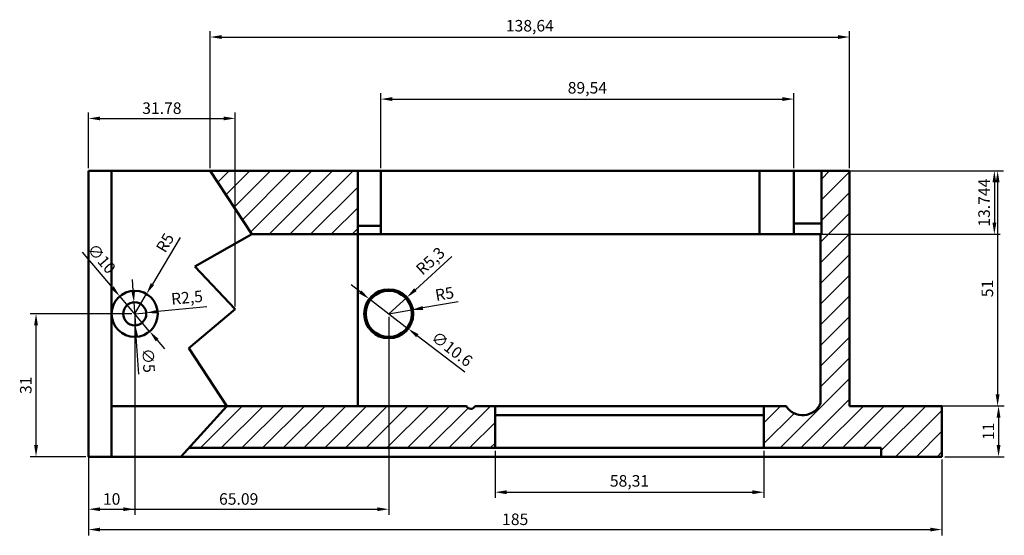
# Model space of a CAD drawing. Units: millimetres. Extents: x 1381 to 2009, y 1325 to 1613.
# Tile 3 of 6: x 1403 to 1617, y 1491 to 1603. Entities that reach past the tile are written whole.
import ezdxf

# ---------------------------------------------------------------- set-up
doc = ezdxf.new("R2010")
doc.units = ezdxf.units.MM
for name, color, linetype, lineweight in [('M-DIMS', 2, 'Continuous', 25), ('M-HATC', 8, 'Continuous', 18), ('M-OUTL', 7, 'Continuous', 50)]:
    doc.layers.add(name, color=color, linetype=linetype, lineweight=lineweight)
doc.styles.get("Standard").update_dxf_attribs({"font": 'arial.ttf'})
doc.dimstyles.new('ISO-25', dxfattribs={"dimtxt": 2.5, "dimasz": 2.5, "dimexe": 1.25, "dimexo": 0.625, "dimtad": 1, "dimtxsty": 'Standard', "dimcen": 2.5, "dimadec": 0, "dimazin": 0, "dimtfac": 1, "dimtmove": 0, "dimatfit": 3, "dimfxl": 1, "dimarcsym": 0})

# ---------------------------------------------------------------- blocks, each defined once
blk = doc.blocks.new('*D68')
at = {"layer": 'Defpoints', "color": 0, "transparency": 16777216}
for p in [(1418.36, 1508.05), (1603.36, 1508.05), (1603.36, 1492.23)]:
    blk.add_point(p, dxfattribs=at)
at = {"layer": 'M-DIMS', "color": 0, "lineweight": -2, "transparency": 16777216}
for p, q in [((1418.36, 1507.42), (1418.36, 1490.98)), ((1603.36, 1507.42), (1603.36, 1490.98)), ((1420.86, 1492.23), (1600.86, 1492.23))]:
    blk.add_line(p, q, dxfattribs=at)
at = {"layer": 'M-DIMS', "color": 0, "transparency": 16777216}
for points in [[(1420.86, 1492.65), (1420.86, 1491.82), (1418.36, 1492.23)], [(1600.86, 1492.65), (1600.86, 1491.82), (1603.36, 1492.23)]]:
    blk.add_solid(points, dxfattribs=at)
at = {"layer": 'M-DIMS', "color": 0, "transparency": 16777216, "insert": (1510.86, 1494.14), "char_height": 2.5, "attachment_point": 5}
blk.add_mtext('185', dxfattribs=at)
blk = doc.blocks.new('*D69')
at = {"layer": 'Defpoints', "color": 0, "transparency": 16777216}
for p in [(1603.36, 1519.05), (1603.36, 1508.05), (1615.67, 1508.05)]:
    blk.add_point(p, dxfattribs=at)
at = {"layer": 'M-DIMS', "color": 0, "lineweight": -2, "transparency": 16777216}
for p, q in [((1603.99, 1519.05), (1616.92, 1519.05)), ((1615.67, 1516.55), (1615.67, 1510.55)), ((1603.99, 1508.05), (1616.92, 1508.05))]:
    blk.add_line(p, q, dxfattribs=at)
at = {"layer": 'M-DIMS', "color": 0, "transparency": 16777216}
for points in [[(1615.25, 1516.55), (1616.09, 1516.55), (1615.67, 1519.05)], [(1615.25, 1510.55), (1616.09, 1510.55), (1615.67, 1508.05)]]:
    blk.add_solid(points, dxfattribs=at)
at = {"layer": 'M-DIMS', "color": 0, "transparency": 16777216, "insert": (1613.79, 1513.55), "char_height": 2.5, "attachment_point": 5, "rotation": 90}
blk.add_mtext('11', dxfattribs=at)
blk = doc.blocks.new('*D70')
at = {"layer": 'Defpoints', "color": 0, "transparency": 16777216}
for p in [(1583.36, 1570.05), (1583.36, 1519.05), (1615.47, 1519.05)]:
    blk.add_point(p, dxfattribs=at)
at = {"layer": 'M-DIMS', "color": 0, "lineweight": -2, "transparency": 16777216}
for p, q in [((1583.99, 1570.05), (1616.72, 1570.05)), ((1615.47, 1567.55), (1615.47, 1521.55)), ((1583.99, 1519.05), (1616.72, 1519.05))]:
    blk.add_line(p, q, dxfattribs=at)
at = {"layer": 'M-DIMS', "color": 0, "transparency": 16777216}
for points in [[(1615.05, 1567.55), (1615.89, 1567.55), (1615.47, 1570.05)], [(1615.05, 1521.55), (1615.89, 1521.55), (1615.47, 1519.05)]]:
    blk.add_solid(points, dxfattribs=at)
at = {"layer": 'M-DIMS', "color": 0, "transparency": 16777216, "insert": (1613.57, 1544.55), "char_height": 2.5, "attachment_point": 5, "rotation": 90}
blk.add_mtext('51', dxfattribs=at)
blk = doc.blocks.new('*D71')
at = {"layer": 'Defpoints', "color": 0, "transparency": 16777216}
for p in [(1583.36, 1599.11), (1444.72, 1570.05), (1583.36, 1570.05)]:
    blk.add_point(p, dxfattribs=at)
at = {"layer": 'M-DIMS', "color": 0, "lineweight": -2, "transparency": 16777216}
for p, q in [((1444.72, 1570.67), (1444.72, 1600.36)), ((1583.36, 1570.67), (1583.36, 1600.36)), ((1447.22, 1599.11), (1580.86, 1599.11))]:
    blk.add_line(p, q, dxfattribs=at)
at = {"layer": 'M-DIMS', "color": 0, "transparency": 16777216}
for points in [[(1447.22, 1599.53), (1447.22, 1598.69), (1444.72, 1599.11)], [(1580.86, 1599.53), (1580.86, 1598.69), (1583.36, 1599.11)]]:
    blk.add_solid(points, dxfattribs=at)
at = {"layer": 'M-DIMS', "color": 0, "transparency": 16777216, "insert": (1514.04, 1601.24), "char_height": 2.5, "attachment_point": 5}
blk.add_mtext('138,64', dxfattribs=at)
blk = doc.blocks.new('*D72')
at = {"layer": 'Defpoints', "color": 0, "transparency": 16777216}
for p in [(1571.28, 1585.65), (1481.73, 1570.05), (1571.28, 1570.05)]:
    blk.add_point(p, dxfattribs=at)
at = {"layer": 'M-DIMS', "color": 0, "lineweight": -2, "transparency": 16777216}
for p, q in [((1481.73, 1570.67), (1481.73, 1586.9)), ((1571.28, 1570.67), (1571.28, 1586.9)), ((1484.23, 1585.65), (1568.78, 1585.65))]:
    blk.add_line(p, q, dxfattribs=at)
at = {"layer": 'M-DIMS', "color": 0, "transparency": 16777216}
for points in [[(1484.23, 1586.07), (1484.23, 1585.23), (1481.73, 1585.65)], [(1568.78, 1586.07), (1568.78, 1585.23), (1571.28, 1585.65)]]:
    blk.add_solid(points, dxfattribs=at)
at = {"layer": 'M-DIMS', "color": 0, "transparency": 16777216, "insert": (1526.51, 1587.78), "char_height": 2.5, "attachment_point": 5}
blk.add_mtext('89,54', dxfattribs=at)
blk = doc.blocks.new('*D73')
at = {"layer": 'Defpoints', "color": 0, "transparency": 16777216}
for p in [(1506.5, 1509.96), (1564.81, 1509.96), (1564.81, 1500.34)]:
    blk.add_point(p, dxfattribs=at)
at = {"layer": 'M-DIMS', "color": 0, "lineweight": -2, "transparency": 16777216}
for p, q in [((1506.5, 1509.34), (1506.5, 1499.09)), ((1564.81, 1509.34), (1564.81, 1499.09)), ((1509, 1500.34), (1562.31, 1500.34))]:
    blk.add_line(p, q, dxfattribs=at)
at = {"layer": 'M-DIMS', "color": 0, "transparency": 16777216}
for points in [[(1509, 1500.75), (1509, 1499.92), (1506.5, 1500.34)], [(1562.31, 1500.75), (1562.31, 1499.92), (1564.81, 1500.34)]]:
    blk.add_solid(points, dxfattribs=at)
at = {"layer": 'M-DIMS', "color": 0, "transparency": 16777216, "insert": (1535.65, 1502.47), "char_height": 2.5, "attachment_point": 5}
blk.add_mtext('58,31', dxfattribs=at)
blk = doc.blocks.new('*D74')
at = {"layer": 'Defpoints', "color": 0, "transparency": 16777216}
for p in [(1487.37, 1542.61), (1483.45, 1539.05)]:
    blk.add_point(p, dxfattribs=at)
at = {"layer": 'M-DIMS', "color": 0, "lineweight": -2, "transparency": 16777216}
for p, q in [((1497.14, 1551.48), (1489.22, 1544.29)), ((1483.45, 1539.05), (1487.37, 1542.61))]:
    blk.add_line(p, q, dxfattribs=at)
at = {"layer": 'M-DIMS', "color": 0, "transparency": 16777216}
blk.add_solid([(1488.94, 1544.6), (1489.5, 1543.98), (1487.37, 1542.61)], dxfattribs=at)
at = {"layer": 'M-DIMS', "color": 0, "transparency": 16777216, "insert": (1492.68, 1550.3), "char_height": 2.5, "attachment_point": 5, "rotation": 42.236}
blk.add_mtext('R5,3', dxfattribs=at)
blk = doc.blocks.new('*D75')
at = {"layer": 'Defpoints', "color": 0, "transparency": 16777216}
for p in [(1488.38, 1539.9), (1483.45, 1539.05)]:
    blk.add_point(p, dxfattribs=at)
at = {"layer": 'M-DIMS', "color": 0, "lineweight": -2, "transparency": 16777216}
for p, q in [((1498.53, 1541.65), (1490.84, 1540.32)), ((1483.45, 1539.05), (1488.38, 1539.9))]:
    blk.add_line(p, q, dxfattribs=at)
at = {"layer": 'M-DIMS', "color": 0, "transparency": 16777216}
blk.add_solid([(1490.77, 1540.73), (1490.91, 1539.91), (1488.38, 1539.9)], dxfattribs=at)
at = {"layer": 'M-DIMS', "color": 0, "transparency": 16777216, "insert": (1495.59, 1543.07), "char_height": 2.5, "attachment_point": 5, "rotation": 9.7906}
blk.add_mtext('R5', dxfattribs=at)
blk = doc.blocks.new('*D76')
at = {"layer": 'Defpoints', "color": 0, "transparency": 16777216}
for p in [(1430.91, 1543.35), (1428.36, 1539.05)]:
    blk.add_point(p, dxfattribs=at)
at = {"layer": 'M-DIMS', "color": 0, "lineweight": -2, "transparency": 16777216}
for p, q in [((1438.2, 1555.62), (1432.19, 1545.5)), ((1428.36, 1539.05), (1430.91, 1543.35))]:
    blk.add_line(p, q, dxfattribs=at)
at = {"layer": 'M-DIMS', "color": 0, "transparency": 16777216}
blk.add_solid([(1431.83, 1545.71), (1432.55, 1545.28), (1430.91, 1543.35)], dxfattribs=at)
at = {"layer": 'M-DIMS', "color": 0, "transparency": 16777216, "insert": (1435.22, 1554.31), "char_height": 2.5, "attachment_point": 5, "rotation": 59.311}
blk.add_mtext('R5', dxfattribs=at)
blk = doc.blocks.new('*D77')
at = {"layer": 'Defpoints', "color": 0, "transparency": 16777216}
for p in [(1428.36, 1539.05), (1430.85, 1539.28)]:
    blk.add_point(p, dxfattribs=at)
at = {"layer": 'M-DIMS', "color": 0, "lineweight": -2, "transparency": 16777216}
for p, q in [((1444, 1540.53), (1433.34, 1539.52)), ((1428.36, 1539.05), (1430.85, 1539.28))]:
    blk.add_line(p, q, dxfattribs=at)
at = {"layer": 'M-DIMS', "color": 0, "transparency": 16777216}
blk.add_solid([(1433.3, 1539.93), (1433.38, 1539.1), (1430.85, 1539.28)], dxfattribs=at)
at = {"layer": 'M-DIMS', "color": 0, "transparency": 16777216, "insert": (1439.72, 1542.26), "char_height": 2.5, "attachment_point": 5, "rotation": 5.4126}
blk.add_mtext('R2,5', dxfattribs=at)
blk = doc.blocks.new('*D78')
at = {"layer": 'Defpoints', "color": 0, "transparency": 16777216}
for p in [(1428.36, 1539.05), (1418.36, 1508.05), (1428.36, 1496.65)]:
    blk.add_point(p, dxfattribs=at)
at = {"layer": 'M-DIMS', "color": 0, "lineweight": -2, "transparency": 16777216}
for p, q in [((1428.36, 1538.42), (1428.36, 1495.4)), ((1418.36, 1507.42), (1418.36, 1495.4)), ((1420.86, 1496.65), (1425.86, 1496.65))]:
    blk.add_line(p, q, dxfattribs=at)
at = {"layer": 'M-DIMS', "color": 0, "transparency": 16777216}
for points in [[(1420.86, 1497.06), (1420.86, 1496.23), (1418.36, 1496.65)], [(1425.86, 1497.06), (1425.86, 1496.23), (1428.36, 1496.65)]]:
    blk.add_solid(points, dxfattribs=at)
at = {"layer": 'M-DIMS', "color": 0, "transparency": 16777216, "insert": (1423.36, 1498.55), "char_height": 2.5, "attachment_point": 5}
blk.add_mtext('10', dxfattribs=at)
blk = doc.blocks.new('*D79')
at = {"layer": 'Defpoints', "color": 0, "transparency": 16777216}
for p in [(1406.96, 1539.05), (1428.36, 1539.05), (1418.36, 1508.05)]:
    blk.add_point(p, dxfattribs=at)
at = {"layer": 'M-DIMS', "color": 0, "lineweight": -2, "transparency": 16777216}
for p, q in [((1427.74, 1539.05), (1405.71, 1539.05)), ((1406.96, 1510.55), (1406.96, 1536.55)), ((1417.74, 1508.05), (1405.71, 1508.05))]:
    blk.add_line(p, q, dxfattribs=at)
at = {"layer": 'M-DIMS', "color": 0, "transparency": 16777216}
for points in [[(1406.55, 1536.55), (1407.38, 1536.55), (1406.96, 1539.05)], [(1406.55, 1510.55), (1407.38, 1510.55), (1406.96, 1508.05)]]:
    blk.add_solid(points, dxfattribs=at)
at = {"layer": 'M-DIMS', "color": 0, "transparency": 16777216, "insert": (1405.06, 1523.55), "char_height": 2.5, "attachment_point": 5, "rotation": 90}
blk.add_mtext('31', dxfattribs=at)
blk = doc.blocks.new('*D80')
at = {"layer": 'Defpoints', "color": 0, "transparency": 16777216}
for p in [(1418.36, 1570.05), (1483.45, 1539.05), (1483.45, 1496.65)]:
    blk.add_point(p, dxfattribs=at)
at = {"layer": 'M-DIMS', "color": 0, "lineweight": -2, "transparency": 16777216}
for p, q in [((1418.36, 1569.42), (1418.36, 1495.4)), ((1483.45, 1538.42), (1483.45, 1495.4)), ((1420.86, 1496.65), (1480.95, 1496.65))]:
    blk.add_line(p, q, dxfattribs=at)
at = {"layer": 'M-DIMS', "color": 0, "transparency": 16777216}
for points in [[(1420.86, 1497.06), (1420.86, 1496.23), (1418.36, 1496.65)], [(1480.95, 1497.06), (1480.95, 1496.23), (1483.45, 1496.65)]]:
    blk.add_solid(points, dxfattribs=at)
at = {"layer": 'M-DIMS', "color": 0, "transparency": 16777216, "insert": (1450.91, 1498.55), "char_height": 2.5, "attachment_point": 5}
blk.add_mtext('65.09', dxfattribs=at)
blk = doc.blocks.new('*D81')
at = {"layer": 'Defpoints', "color": 0, "transparency": 16777216}
for p in [(1476.73, 1570.05), (1476.73, 1556.3), (1614.76, 1556.3)]:
    blk.add_point(p, dxfattribs=at)
at = {"layer": 'M-DIMS', "color": 0, "lineweight": -2, "transparency": 16777216}
for p, q in [((1477.36, 1570.05), (1616.01, 1570.05)), ((1614.76, 1567.55), (1614.76, 1558.8)), ((1477.36, 1556.3), (1616.01, 1556.3))]:
    blk.add_line(p, q, dxfattribs=at)
at = {"layer": 'M-DIMS', "color": 0, "transparency": 16777216}
for points in [[(1614.35, 1567.55), (1615.18, 1567.55), (1614.76, 1570.05)], [(1614.35, 1558.8), (1615.18, 1558.8), (1614.76, 1556.3)]]:
    blk.add_solid(points, dxfattribs=at)
at = {"layer": 'M-DIMS', "color": 0, "transparency": 16777216, "insert": (1612.86, 1563.17), "char_height": 2.5, "attachment_point": 5, "rotation": 90}
blk.add_mtext('13.744', dxfattribs=at)
blk = doc.blocks.new('*D82')
at = {"layer": 'Defpoints', "color": 0, "transparency": 16777216}
for p in [(1450.14, 1581.45), (1418.36, 1570.05), (1450.14, 1540.03)]:
    blk.add_point(p, dxfattribs=at)
at = {"layer": 'M-DIMS', "color": 0, "lineweight": -2, "transparency": 16777216}
for p, q in [((1418.36, 1570.67), (1418.36, 1582.7)), ((1450.14, 1540.65), (1450.14, 1582.7)), ((1420.86, 1581.45), (1447.64, 1581.45))]:
    blk.add_line(p, q, dxfattribs=at)
at = {"layer": 'M-DIMS', "color": 0, "transparency": 16777216}
for points in [[(1420.86, 1581.86), (1420.86, 1581.03), (1418.36, 1581.45)], [(1447.64, 1581.86), (1447.64, 1581.03), (1450.14, 1581.45)]]:
    blk.add_solid(points, dxfattribs=at)
at = {"layer": 'M-DIMS', "color": 0, "transparency": 16777216, "insert": (1434.25, 1583.35), "char_height": 2.5, "attachment_point": 5}
blk.add_mtext('31.78', dxfattribs=at)
blk = doc.blocks.new('*D104')
at = {"layer": 'Defpoints', "color": 0, "transparency": 16777216}
for p in [(1425.12, 1542.85), (1431.6, 1535.24)]:
    blk.add_point(p, dxfattribs=at)
at = {"layer": 'M-DIMS', "color": 0, "lineweight": -2, "transparency": 16777216}
for p, q in [((1416.99, 1552.4), (1423.5, 1544.76)), ((1431.6, 1535.24), (1425.12, 1542.85)), ((1433.23, 1533.34), (1434.85, 1531.43))]:
    blk.add_line(p, q, dxfattribs=at)
at = {"layer": 'M-DIMS', "color": 0, "transparency": 16777216}
for points in [[(1423.82, 1545.03), (1423.18, 1544.49), (1425.12, 1542.85)], [(1433.54, 1533.61), (1432.91, 1533.07), (1431.6, 1535.24)]]:
    blk.add_solid(points, dxfattribs=at)
at = {"layer": 'M-DIMS', "color": 0, "transparency": 16777216, "insert": (1420.93, 1550.81), "char_height": 2.5, "attachment_point": 5, "rotation": 310.4242}
blk.add_mtext('∅10', dxfattribs=at)
blk = doc.blocks.new('*D105')
at = {"layer": 'Defpoints', "color": 0, "transparency": 16777216}
for p in [(1428.19, 1541.54), (1428.53, 1536.55)]:
    blk.add_point(p, dxfattribs=at)
at = {"layer": 'M-DIMS', "color": 0, "lineweight": -2, "transparency": 16777216}
for p, q in [((1428.03, 1544.03), (1427.86, 1546.53)), ((1428.19, 1541.54), (1428.53, 1536.55)), ((1429.24, 1525.95), (1428.7, 1534.06))]:
    blk.add_line(p, q, dxfattribs=at)
at = {"layer": 'M-DIMS', "color": 0, "transparency": 16777216}
for points in [[(1428.44, 1544.06), (1427.61, 1544.01), (1428.19, 1541.54)], [(1429.11, 1534.09), (1428.28, 1534.03), (1428.53, 1536.55)]]:
    blk.add_solid(points, dxfattribs=at)
at = {"layer": 'M-DIMS', "color": 0, "transparency": 16777216, "insert": (1431.02, 1528.89), "char_height": 2.5, "attachment_point": 5, "rotation": 273.8557}
blk.add_mtext('∅5', dxfattribs=at)
blk = doc.blocks.new('*D106')
at = {"layer": 'Defpoints', "color": 0, "transparency": 16777216}
for p in [(1479.24, 1542.27), (1487.66, 1535.82)]:
    blk.add_point(p, dxfattribs=at)
at = {"layer": 'M-DIMS', "color": 0, "lineweight": -2, "transparency": 16777216}
for p, q in [((1477.26, 1543.79), (1475.27, 1545.31)), ((1479.24, 1542.27), (1487.66, 1535.82)), ((1499.93, 1526.42), (1489.64, 1534.3))]:
    blk.add_line(p, q, dxfattribs=at)
at = {"layer": 'M-DIMS', "color": 0, "transparency": 16777216}
for points in [[(1477.51, 1544.12), (1477, 1543.46), (1479.24, 1542.27)], [(1489.89, 1534.63), (1489.39, 1533.97), (1487.66, 1535.82)]]:
    blk.add_solid(points, dxfattribs=at)
at = {"layer": 'M-DIMS', "color": 0, "transparency": 16777216, "insert": (1496.98, 1531.16), "char_height": 2.5, "attachment_point": 5, "rotation": 322.5392}
blk.add_mtext('∅10.6', dxfattribs=at)

msp = doc.modelspace()

# ---------------------------------------------------------------- hatches: boundary and pattern name
at = {"layer": 'M-HATC'}
h = msp.add_hatch(dxfattribs=at)
h.set_pattern_fill('ANSI31', color=256)
h.paths.add_polyline_path([(1506.5017, 1519.0093), (1502.1541, 1519.0093, -0.64754949), (1500.2882, 1519.046), (1448.3621, 1519.046), (1440.0944, 1509.9609), (1506.5017, 1509.9609)])
h.paths.add_polyline_path([(1603.3621, 1519.046), (1583.3621, 1519.046), (1583.3621, 1570.046), (1577.2775, 1570.046), (1577.2775, 1556.3016), (1577.0745, 1556.3016), (1577.0745, 1519.6796, -0.61519467), (1569.6085, 1519.0093), (1564.8072, 1519.0093), (1564.8072, 1509.9609), (1590.2309, 1509.9609), (1590.2309, 1508.046), (1603.3621, 1508.046)])
h.paths.add_polyline_path([(1476.7341, 1570.046), (1444.7225, 1570.046), (1453.7787, 1556.3016), (1476.7341, 1556.3016)])

# ---------------------------------------------------------------- linework, layer by layer
at = {"layer": 'M-OUTL'}
for p, q in [((1423.3621, 1570.046), (1418.3621, 1570.046)), ((1418.3621, 1570.046), (1418.3621, 1508.046)), ((1583.3621, 1570.046), (1423.3621, 1570.046)), ((1423.3621, 1508.046), (1423.3621, 1570.046)), ((1453.7787, 1556.3016), (1444.7225, 1570.046)), ((1476.7341, 1570.046), (1476.7341, 1556.3016)), ((1481.7341, 1556.3016), (1481.7341, 1570.046)), ((1563.8534, 1556.3016), (1563.8534, 1570.046)), ((1571.2775, 1570.046), (1571.2775, 1556.3016)), ((1577.2775, 1556.3016), (1577.2775, 1570.046)), ((1583.3621, 1519.046), (1583.3621, 1570.046)), ((1571.2775, 1558.6222), (1577.2775, 1558.6222)), ((1476.7341, 1558.17), (1481.7341, 1558.17)), ((1441.4165, 1549.3267), (1453.7787, 1556.3016)), ((1453.7787, 1556.3016), (1577.0745, 1556.3016)), ((1476.7341, 1556.3016), (1476.7341, 1519.046)), ((1577.0745, 1519.6796), (1577.0745, 1556.3016)), ((1577.0745, 1556.3016), (1577.2775, 1556.3016)), ((1450.1428, 1540.0268), (1441.4165, 1549.3267)), ((1440.1076, 1531.5988), (1450.1428, 1540.0268)), ((1448.3621, 1519.046), (1440.1076, 1531.5988)), ((1423.3621, 1508.046), (1423.3621, 1519.046)), ((1423.3621, 1519.046), (1448.3621, 1519.046)), ((1438.3517, 1508.046), (1448.3621, 1519.046)), ((1448.3621, 1519.046), (1500.2882, 1519.046)), ((1502.1541, 1519.0093), (1569.6085, 1519.0093)), ((1506.5017, 1519.0093), (1506.5017, 1509.9609)), ((1564.8072, 1519.0093), (1564.8072, 1509.9609)), ((1603.3621, 1519.046), (1583.3621, 1519.046)), ((1603.3621, 1508.046), (1603.3621, 1519.046)), ((1506.5017, 1517.0867), (1564.8072, 1517.0867)), ((1440.0944, 1509.9609), (1590.2309, 1509.9609)), ((1590.2309, 1509.9609), (1590.2309, 1508.046)), ((1418.3621, 1508.046), (1423.3621, 1508.046)), ((1423.3621, 1508.046), (1603.3621, 1508.046))]:
    msp.add_line(p, q, dxfattribs=at)
for centre, radius in [((1428.3621, 1539.046), 5), ((1483.4485, 1539.046), 5.3), ((1483.4485, 1539.046), 5), ((1428.3621, 1539.046), 2.5)]:
    msp.add_circle(centre, radius, dxfattribs=at)
for centre, radius, start, end in [((1501.2294, 1519.4459), 1.0226, 203.023774, 334.723993), ((1573.1722, 1521.2302), 4.1991, 211.930871, 338.329303)]:
    msp.add_arc(centre, radius, start, end, dxfattribs=at)

# ---------------------------------------------------------------- dimensions: what is measured, and where the dimension line sits
at = {"layer": 'M-DIMS'}
for base, p1, p2, override, picture, middle in [((1583.3621, 1599.1086), (1444.7225, 1570.046), (1583.3621, 1570.046), {"dimclrd": 0, "dimclre": 0, "dimclrt": 0}, '*D71', (1514.0423, 1601.236)), ((1571.2775, 1585.6488), (1481.7341, 1570.046), (1571.2775, 1570.046), {"dimclrd": 0, "dimclre": 0, "dimclrt": 0}, '*D72', (1526.5058, 1587.7762)), ((1450.1428, 1581.446), (1418.3621, 1570.046), (1450.1428, 1540.0268), {"dimdec": 2, "dimlfac": 1, "dimrnd": 0, "dimzin": 0, "dimdsep": 46, "dimlunit": 2}, '*D82', (1434.2525, 1583.3482)), ((1483.4485, 1496.646), (1418.3621, 1570.046), (1483.4485, 1539.046), {"dimdec": 2, "dimlfac": 1, "dimrnd": 0, "dimzin": 0, "dimdsep": 46, "dimlunit": 2}, '*D80', (1450.9053, 1498.5474)), ((1428.3621, 1496.646), (1418.3621, 1508.046), (1428.3621, 1539.046), {"dimdec": 0, "dimlfac": 1, "dimrnd": 0, "dimzin": 0, "dimdsep": 46, "dimlunit": 2}, '*D78', (1423.3621, 1498.5474)), ((1564.8072, 1500.3379), (1506.5017, 1509.9609), (1564.8072, 1509.9609), {"dimclrd": 0, "dimclre": 0, "dimclrt": 0}, '*D73', (1535.6545, 1502.4653)), ((1603.3621, 1492.2337), (1418.3621, 1508.046), (1603.3621, 1508.046), {"dimclrd": 0, "dimclre": 0, "dimclrt": 0}, '*D68', (1510.8621, 1494.1351))]:
    dim = msp.add_linear_dim(base=base, p1=p1, p2=p2, dimstyle='ISO-25', override=override, dxfattribs=at)
    dim.commit()
    dim.dimension.update_dxf_attribs({"geometry": picture, "text_midpoint": middle})
for base, p1, p2, override, picture, middle in [((1614.7621, 1556.3016), (1476.7341, 1570.046), (1476.7341, 1556.3016), {"dimdec": 3, "dimlfac": 1, "dimrnd": 0, "dimzin": 0, "dimdsep": 46, "dimlunit": 2}, '*D81', (1612.8598, 1563.1738)), ((1615.4706, 1519.046), (1583.3621, 1570.046), (1583.3621, 1519.046), {"dimclrd": 0, "dimclre": 0, "dimclrt": 0}, '*D70', (1613.5692, 1544.546)), ((1406.9621, 1539.046), (1418.3621, 1508.046), (1428.3621, 1539.046), {"dimdec": 0, "dimlfac": 1, "dimrnd": 0, "dimzin": 0, "dimdsep": 46, "dimlunit": 2}, '*D79', (1405.0598, 1523.546)), ((1615.6691, 1508.046), (1603.3621, 1519.046), (1603.3621, 1508.046), {"dimclrd": 0, "dimclre": 0, "dimclrt": 0}, '*D69', (1613.789, 1513.546))]:
    dim = msp.add_linear_dim(base=base, p1=p1, p2=p2, angle=90, dimstyle='ISO-25', override=override, dxfattribs=at)
    dim.commit()
    dim.dimension.update_dxf_attribs({"geometry": picture, "text_midpoint": middle})
dim = msp.add_radius_dim(center=(1428.3621, 1539.046), mpoint=(1430.914, 1543.3457), dimstyle='ISO-25', override={"dimclrd": 0, "dimclre": 0, "dimclrt": 0}, dxfattribs=at)
dim.commit()
dim.dimension.update_dxf_attribs({"geometry": '*D76', "text_midpoint": (1436.8475, 1553.3433), "dimtype": 164})
for p1, p2, picture, middle in [((1431.6043, 1535.2396), (1425.1199, 1542.8523), '*D104', (1419.4322, 1549.5296)), ((1428.194, 1541.5403), (1428.5302, 1536.5516), '*D105', (1429.0557, 1528.7555))]:
    dim = msp.add_diameter_dim_2p(p1=p1, p2=p2, dimstyle='ISO-25', override={"dimdec": 0, "dimlfac": 1, "dimrnd": 0, "dimzin": 0, "dimdsep": 46, "dimlunit": 2}, dxfattribs=at)
    dim.commit()
    dim.dimension.update_dxf_attribs({"geometry": picture, "text_midpoint": middle, "dimtype": 163})
for center, mpoint, picture, middle in [((1483.4485, 1539.046), (1487.3726, 1542.6085), '*D74', (1492.6778, 1550.2985)), ((1428.3621, 1539.046), (1430.851, 1539.2818), '*D77', (1439.7161, 1542.2587)), ((1483.4485, 1539.046), (1488.3757, 1539.8962), '*D75', (1495.5919, 1543.0658))]:
    dim = msp.add_radius_dim(center=center, mpoint=mpoint, dimstyle='ISO-25', override={"dimclrd": 0, "dimclre": 0, "dimclrt": 0}, dxfattribs=at)
    dim.commit()
    dim.dimension.update_dxf_attribs({"geometry": picture, "text_midpoint": middle})
dim = msp.add_diameter_dim_2p(p1=(1479.2415, 1542.2695), p2=(1487.6555, 1535.8224), dimstyle='ISO-25', override={"dimdec": 1, "dimlfac": 1, "dimrnd": 0, "dimzin": 0, "dimdsep": 46, "dimlunit": 2}, dxfattribs=at)
dim.commit()
dim.dimension.update_dxf_attribs({"geometry": '*D106', "text_midpoint": (1495.7766, 1529.5997)})

doc.saveas('drawing.dxf')
